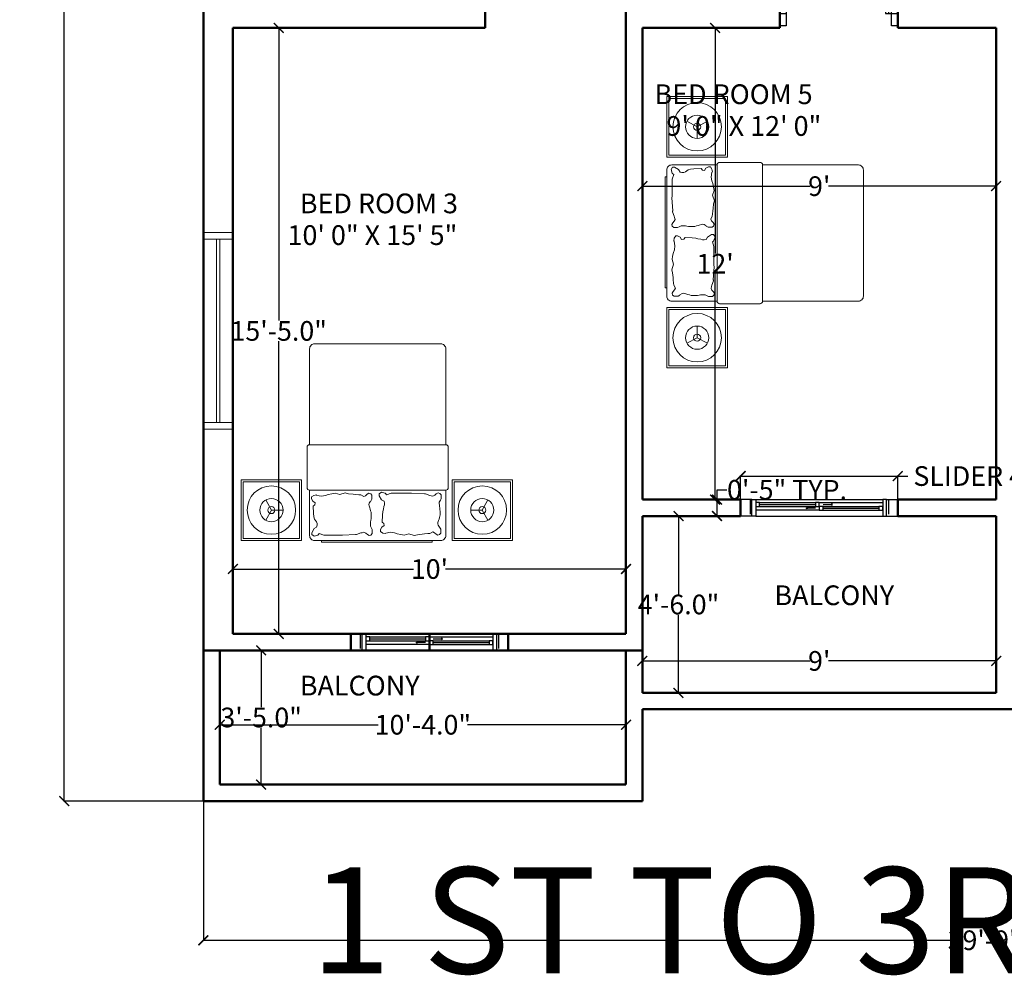
# Model space of a CAD drawing. Units: inches. Extents: x 147 to 1638, y 107 to 941.
# Tile 12 of 17: x 1062 to 1362, y 107 to 398. Entities that reach past the tile are written whole.
import ezdxf

# ---------------------------------------------------------------- set-up
doc = ezdxf.new("R2010")
doc.units = ezdxf.units.IN
doc.header["$MEASUREMENT"] = 0
for name, color, linetype, lineweight in [('A-ANNO-DIMS', 2, 'Continuous', 15), ('A-ANNO-TEXT', 7, 'Continuous', 25), ('A-AREA-IDEN', 7, 'Continuous', 18), ('A-Door', 150, 'Continuous', 25), ('furniture', 50, 'Continuous', 18), ('walls', 7, 'Continuous', 50), ('windows', 3, 'Continuous', 20)]:
    doc.layers.add(name, color=color, linetype=linetype, lineweight=lineweight)
doc.layers.add('A-Glaz', color=92, linetype='Continuous')
doc.layers.add('NT', color=1, linetype='Continuous')
doc.styles.get("Standard").update_dxf_attribs({"font": 'arial.ttf'})
doc.dimstyles.get("Standard").update_dxf_attribs({"dimtxt": 6, "dimasz": 3, "dimexe": 0.18, "dimexo": 0.0625, "dimgap": 0.09, "dimtad": 0, "dimtih": 1, "dimtoh": 1, "dimdec": 1, "dimzin": 0, "dimdsep": 46, "dimlunit": 3, "dimtxsty": 'Standard', "dimblk": 'ARCHTICK', "dimcen": 0.09, "dimadec": 0, "dimazin": 0, "dimtfac": 1, "dimtdec": 1, "dimtofl": 0, "dimtmove": 0, "dimatfit": 3, "dimfxl": 1, "dimtolj": 1, "dimtzin": 0, "dimarcsym": 0})

# ---------------------------------------------------------------- blocks, each defined once
blk = doc.blocks.new('A$C087A3AA9')
at = {"layer": 'A-Door'}
for points in [[(852.6, 94.7), (852.6, 852.6), (805.3, 852.6), (805.3, 94.7)], [(47.4, 94.7), (47.4, 0), (0, 0), (0, 94.7)], [(900, 94.7), (900, 0), (852.6, 0), (852.6, 94.7)]]:
    blk.add_lwpolyline(points, close=True, dxfattribs=at)
at = {"layer": 'A-Glaz'}
blk.add_line((828.9, 852.6), (828.9, 94.7), dxfattribs=at)
at = {"layer": 'NT'}
blk.add_arc((805.3, 94.7), 757.9, 90, 180, dxfattribs=at)
blk = doc.blocks.new('_ArchTick')
at = {"color": 0, "linetype": 'ByBlock', "const_width": 0.15}
blk.add_lwpolyline([(-0.5, -0.5), (0.5, 0.5)], dxfattribs=at)
blk = doc.blocks.new('*D34')
at = {"layer": 'A-ANNO-DIMS', "color": 0, "lineweight": -2, "transparency": 16777216}
for p, q in [((1266.83, 395.72), (1274.16, 395.72)), ((1273.98, 395.72), (1273.98, 326.82)), ((1273.98, 251.72), (1273.98, 320.62)), ((1266.83, 251.72), (1274.16, 251.72))]:
    blk.add_line(p, q, dxfattribs=at)
at = {"layer": 'Defpoints', "color": 0, "lineweight": -2, "transparency": 16777216}
for p in [(1266.77, 395.72), (1266.77, 251.72), (1273.98, 251.72)]:
    blk.add_point(p, dxfattribs=at)
at = {"layer": 'A-ANNO-DIMS', "color": 0, "lineweight": -2, "transparency": 16777216, "xscale": 3, "yscale": 3, "zscale": 3}
for p, rotation in [((1273.98, 395.72), 90), ((1273.98, 251.72), 270)]:
    blk.add_blockref('_ArchTick', p, dxfattribs=dict(at, rotation=rotation))
at = {"layer": 'A-ANNO-DIMS', "color": 0, "transparency": 16777216, "insert": (1273.98, 323.72), "char_height": 6, "attachment_point": 5}
blk.add_mtext("\\A1;12'", dxfattribs=at)
blk = doc.blocks.new('*D35')
at = {"layer": 'A-ANNO-DIMS', "color": 0, "lineweight": -2, "transparency": 16777216}
for p, q in [((1251.77, 336.12), (1251.77, 347.59)), ((1251.77, 347.41), (1302.92, 347.41)), ((1359.77, 347.41), (1308.62, 347.41)), ((1359.77, 336.12), (1359.77, 347.59))]:
    blk.add_line(p, q, dxfattribs=at)
at = {"layer": 'Defpoints', "color": 0, "lineweight": -2, "transparency": 16777216}
for p in [(1359.77, 347.41), (1251.77, 336.06), (1359.77, 336.06)]:
    blk.add_point(p, dxfattribs=at)
at = {"layer": 'A-ANNO-DIMS', "color": 0, "lineweight": -2, "transparency": 16777216, "xscale": 3, "yscale": 3, "zscale": 3, "rotation": 180}
blk.add_blockref('_ArchTick', (1251.77, 347.41), dxfattribs=at)
at = {"layer": 'A-ANNO-DIMS', "color": 0, "lineweight": -2, "transparency": 16777216, "xscale": 3, "yscale": 3, "zscale": 3}
blk.add_blockref('_ArchTick', (1359.77, 347.41), dxfattribs=at)
at = {"layer": 'A-ANNO-DIMS', "color": 0, "transparency": 16777216, "insert": (1305.77, 347.41), "char_height": 6, "attachment_point": 5}
blk.add_mtext("\\A1;9'", dxfattribs=at)
blk = doc.blocks.new('*D63')
at = {"layer": 'A-ANNO-DIMS', "color": 0, "lineweight": -2, "transparency": 16777216}
for p, q in [((1138.96, 395.72), (1140.94, 395.72)), ((1140.76, 395.72), (1140.76, 306.37)), ((1140.76, 210.72), (1140.76, 300.06)), ((1138.96, 210.72), (1140.94, 210.72))]:
    blk.add_line(p, q, dxfattribs=at)
at = {"layer": 'Defpoints', "color": 0, "lineweight": -2, "transparency": 16777216}
for p in [(1138.89, 395.72), (1138.89, 210.72), (1140.76, 210.72)]:
    blk.add_point(p, dxfattribs=at)
at = {"layer": 'A-ANNO-DIMS', "color": 0, "lineweight": -2, "transparency": 16777216, "xscale": 3, "yscale": 3, "zscale": 3}
for p, rotation in [((1140.76, 395.72), 90), ((1140.76, 210.72), 270)]:
    blk.add_blockref('_ArchTick', p, dxfattribs=dict(at, rotation=rotation))
at = {"layer": 'A-ANNO-DIMS', "color": 0, "transparency": 16777216, "insert": (1140.76, 303.22), "char_height": 6, "attachment_point": 5}
blk.add_mtext('\\A1;15\'-5.0"', dxfattribs=at)
blk = doc.blocks.new('*D64')
at = {"layer": 'A-ANNO-DIMS', "color": 0, "lineweight": -2, "transparency": 16777216}
for p, q in [((1126.77, 232.37), (1126.77, 230.36)), ((1246.77, 232.37), (1246.77, 230.36)), ((1126.77, 230.54), (1181.87, 230.54)), ((1246.77, 230.54), (1191.67, 230.54))]:
    blk.add_line(p, q, dxfattribs=at)
at = {"layer": 'Defpoints', "color": 0, "lineweight": -2, "transparency": 16777216}
for p in [(1126.77, 232.43), (1246.77, 232.43), (1246.77, 230.54)]:
    blk.add_point(p, dxfattribs=at)
at = {"layer": 'A-ANNO-DIMS', "color": 0, "lineweight": -2, "transparency": 16777216, "xscale": 3, "yscale": 3, "zscale": 3, "rotation": 180}
blk.add_blockref('_ArchTick', (1126.77, 230.54), dxfattribs=at)
at = {"layer": 'A-ANNO-DIMS', "color": 0, "lineweight": -2, "transparency": 16777216, "xscale": 3, "yscale": 3, "zscale": 3}
blk.add_blockref('_ArchTick', (1246.77, 230.54), dxfattribs=at)
at = {"layer": 'A-ANNO-DIMS', "color": 0, "transparency": 16777216, "insert": (1186.77, 230.54), "char_height": 6, "attachment_point": 5}
blk.add_mtext("\\A1;10'", dxfattribs=at)
blk = doc.blocks.new('*D67')
at = {"layer": 'A-ANNO-DIMS', "color": 0, "lineweight": -2, "transparency": 16777216}
for p, q in [((1122.77, 185.16), (1122.77, 182.83)), ((1246.77, 185.16), (1246.77, 182.83)), ((1122.77, 183.01), (1171.16, 183.01)), ((1246.77, 183.01), (1198.38, 183.01))]:
    blk.add_line(p, q, dxfattribs=at)
at = {"layer": 'Defpoints', "color": 0, "lineweight": -2, "transparency": 16777216}
for p in [(1122.77, 185.22), (1246.77, 185.22), (1246.77, 183.01)]:
    blk.add_point(p, dxfattribs=at)
at = {"layer": 'A-ANNO-DIMS', "color": 0, "lineweight": -2, "transparency": 16777216, "xscale": 3, "yscale": 3, "zscale": 3, "rotation": 180}
blk.add_blockref('_ArchTick', (1122.77, 183.01), dxfattribs=at)
at = {"layer": 'A-ANNO-DIMS', "color": 0, "lineweight": -2, "transparency": 16777216, "xscale": 3, "yscale": 3, "zscale": 3}
blk.add_blockref('_ArchTick', (1246.77, 183.01), dxfattribs=at)
at = {"layer": 'A-ANNO-DIMS', "color": 0, "transparency": 16777216, "insert": (1184.77, 183.01), "char_height": 6, "attachment_point": 5}
blk.add_mtext('\\A1;10\'-4.0"', dxfattribs=at)
blk = doc.blocks.new('*D68')
at = {"layer": 'A-ANNO-DIMS', "color": 0, "lineweight": -2, "transparency": 16777216}
for p, q in [((1132.43, 205.72), (1135.58, 205.72)), ((1135.4, 205.72), (1135.4, 188.37)), ((1135.4, 164.72), (1135.4, 182.06)), ((1132.43, 164.72), (1135.58, 164.72))]:
    blk.add_line(p, q, dxfattribs=at)
at = {"layer": 'Defpoints', "color": 0, "lineweight": -2, "transparency": 16777216}
for p in [(1132.37, 205.72), (1132.37, 164.72), (1135.4, 164.72)]:
    blk.add_point(p, dxfattribs=at)
at = {"layer": 'A-ANNO-DIMS', "color": 0, "lineweight": -2, "transparency": 16777216, "xscale": 3, "yscale": 3, "zscale": 3}
for p, rotation in [((1135.4, 205.72), 90), ((1135.4, 164.72), 270)]:
    blk.add_blockref('_ArchTick', p, dxfattribs=dict(at, rotation=rotation))
at = {"layer": 'A-ANNO-DIMS', "color": 0, "transparency": 16777216, "insert": (1135.4, 185.22), "char_height": 6, "attachment_point": 5}
blk.add_mtext('\\A1;3\'-5.0"', dxfattribs=at)
blk = doc.blocks.new('MAT-P14')
for p, q in [((-1.3369, 1.348), (-1.3369, 1.948)), ((-1.3369, 1.948), (-0.7369, 1.948)), ((-1.3169, 1.928), (-0.7569, 1.928)), ((-1.3169, 1.368), (-1.3169, 1.928)), ((-0.7569, 1.368), (-0.7569, 1.928)), ((-0.7369, 1.348), (-0.7369, 1.948)), ((0.625, 1.95), (-0.625, 1.95)), ((0.7534, 1.348), (0.7534, 1.948)), ((1.3534, 1.948), (0.7534, 1.948)), ((1.3334, 1.928), (0.7734, 1.928)), ((0.7734, 1.368), (0.7734, 1.928)), ((1.3334, 1.368), (1.3334, 1.928)), ((1.3534, 1.348), (1.3534, 1.948)), ((-1.0369, 1.648), (-1.0913, 1.7493)), ((1.0534, 1.648), (1.1078, 1.7493)), ((-1.0369, 1.648), (-1.0913, 1.5467)), ((-1.0369, 1.648), (-0.9219, 1.648)), ((1.0534, 1.648), (0.9384, 1.648)), ((1.0534, 1.648), (1.1078, 1.5467)), ((-1.3169, 1.368), (-0.7569, 1.368)), ((1.3334, 1.368), (0.7734, 1.368)), ((-1.3369, 1.348), (-0.7369, 1.348)), ((1.3534, 1.348), (0.7534, 1.348))]:
    blk.add_line(p, q)
blk.add_lwpolyline([(-0.5417, 1.95), (-0.5417, 1.9665), (0.5583, 1.9665), (0.5583, 1.95)], close=True)
for points in [[(-0.675, 1.45), (-0.675, 1.9, -0.414214), (-0.625, 1.95), (0.625, 1.95, -0.414214), (0.675, 1.9), (0.675, 1.45)], [(-0.675, 1, -0.414214), (-0.7, 1.025), (-0.7, 1.425, -0.414214), (-0.675, 1.45), (0.675, 1.45, -0.414214), (0.7, 1.425), (0.7, 1.025, -0.414214), (0.675, 1)], [(-0.625, 0, -0.414214), (-0.675, 0.05), (-0.675, 1), (0.675, 1), (0.675, 0.05, -0.414214), (0.625, 0)]]:
    blk.add_lwpolyline(points, format="xyb", close=True)
for points in [[(-0.6142, 1.8182), (-0.6262, 1.8377), (-0.6262, 1.8767), (-0.6142, 1.8914), (-0.5964, 1.8963), (-0.5785, 1.8865), (-0.563, 1.8719), (-0.5451, 1.8633), (-0.5157, 1.879), (-0.4966, 1.8816), (-0.4647, 1.8842), (-0.4393, 1.8868), (-0.3947, 1.892), (-0.3629, 1.8999), (-0.3094, 1.8823), (-0.2619, 1.8969), (-0.23, 1.8916), (-0.1918, 1.8838), (-0.1664, 1.8734), (-0.1282, 1.8682), (-0.0818, 1.8753), (-0.0758, 1.8802), (-0.052, 1.8753), (-0.0281, 1.8607), (-0.0281, 1.8412), (-0.0401, 1.8168), (-0.0639, 1.8022), (-0.0598, 1.781), (-0.0431, 1.7682), (-0.0463, 1.6973), (-0.0502, 1.6621), (-0.0561, 1.6397), (-0.0619, 1.6125), (-0.0678, 1.5965), (-0.0678, 1.5789), (-0.0631, 1.5599), (-0.0393, 1.5453), (-0.0147, 1.5053), (-0.0147, 1.4858), (-0.0385, 1.4711), (-0.0751, 1.4819), (-0.081, 1.4868), (-0.087, 1.4965), (-0.1344, 1.4812), (-0.3042, 1.4815), (-0.3178, 1.4815), (-0.3355, 1.4791), (-0.4636, 1.4878), (-0.4672, 1.4865), (-0.4732, 1.4863), (-0.5167, 1.5026), (-0.5299, 1.5053), (-0.5478, 1.5102), (-0.5656, 1.5015), (-0.5812, 1.4869), (-0.599, 1.4772), (-0.6169, 1.482), (-0.6288, 1.4967), (-0.6288, 1.5357), (-0.6229, 1.5503), (-0.611, 1.5698), (-0.6136, 1.6138), (-0.6149, 1.6269), (-0.6176, 1.6443), (-0.6189, 1.6595), (-0.6202, 1.6748), (-0.6202, 1.6955), (-0.6176, 1.7075), (-0.6136, 1.7227), (-0.6083, 1.7391), (-0.6043, 1.75), (-0.5976, 1.7707), (-0.5963, 1.7848), (-0.6003, 1.7979), (-0.6136, 1.8186)], [(0.0694, 1.5591), (0.0575, 1.5396), (0.0575, 1.5006), (0.0694, 1.4859), (0.0873, 1.481), (0.1052, 1.4908), (0.1207, 1.5054), (0.1386, 1.514), (0.168, 1.4983), (0.1871, 1.4957), (0.2189, 1.4931), (0.2444, 1.4905), (0.289, 1.4853), (0.3208, 1.4774), (0.3742, 1.495), (0.4218, 1.4804), (0.4536, 1.4857), (0.4918, 1.4935), (0.5173, 1.5039), (0.5555, 1.5091), (0.6019, 1.502), (0.6079, 1.4971), (0.6317, 1.502), (0.6555, 1.5166), (0.6555, 1.5361), (0.6436, 1.5605), (0.6198, 1.5751), (0.6239, 1.5963), (0.6405, 1.6091), (0.6373, 1.68), (0.6334, 1.7152), (0.6276, 1.7376), (0.6063, 1.7648), (0.6005, 1.7808), (0.6005, 1.7984), (0.6051, 1.8174), (0.6289, 1.832), (0.6536, 1.872), (0.6536, 1.8915), (0.6298, 1.9062), (0.5932, 1.8954), (0.5872, 1.8905), (0.5813, 1.8808), (0.5338, 1.8961), (0.3795, 1.8958), (0.3658, 1.8958), (0.3482, 1.8982), (0.2201, 1.8895), (0.2165, 1.8908), (0.2104, 1.891), (0.1669, 1.8747), (0.1538, 1.872), (0.1359, 1.8671), (0.118, 1.8758), (0.1025, 1.8904), (0.0846, 1.9001), (0.0667, 1.8953), (0.0548, 1.8806), (0.0548, 1.8416), (0.0608, 1.827), (0.0727, 1.8075), (0.0701, 1.7635), (0.0688, 1.7504), (0.0661, 1.733), (0.0648, 1.7178), (0.0634, 1.7025), (0.0634, 1.6818), (0.0661, 1.6698), (0.0701, 1.6546), (0.0754, 1.6382), (0.0794, 1.6273), (0.086, 1.6066), (0.0874, 1.5925), (0.0834, 1.5794), (0.0701, 1.5587)]]:
    blk.add_lwpolyline(points)
for centre, radius in [((-1.0369, 1.648), 0.24), ((1.0534, 1.648), 0.24), ((-1.0369, 1.648), 0.115), ((1.0534, 1.648), 0.115), ((-1.0369, 1.648), 0.035), ((1.0534, 1.648), 0.035)]:
    blk.add_circle(centre, radius)
blk = doc.blocks.new('*D83')
at = {"layer": 'A-ANNO-DIMS', "color": 0, "lineweight": -2, "transparency": 16777216}
for p, q in [((1261.96, 246.72), (1262.99, 246.72)), ((1262.81, 246.72), (1262.81, 222.87)), ((1262.81, 192.72), (1262.81, 216.56)), ((1261.96, 192.72), (1262.99, 192.72))]:
    blk.add_line(p, q, dxfattribs=at)
at = {"layer": 'Defpoints', "color": 0, "lineweight": -2, "transparency": 16777216}
for p in [(1261.89, 246.72), (1261.89, 192.72), (1262.81, 192.72)]:
    blk.add_point(p, dxfattribs=at)
at = {"layer": 'A-ANNO-DIMS', "color": 0, "lineweight": -2, "transparency": 16777216, "xscale": 3, "yscale": 3, "zscale": 3}
for p, rotation in [((1262.81, 246.72), 90), ((1262.81, 192.72), 270)]:
    blk.add_blockref('_ArchTick', p, dxfattribs=dict(at, rotation=rotation))
at = {"layer": 'A-ANNO-DIMS', "color": 0, "transparency": 16777216, "insert": (1262.81, 219.72), "char_height": 6, "attachment_point": 5}
blk.add_mtext('\\A1;4\'-6.0"', dxfattribs=at)
blk = doc.blocks.new('*D84')
at = {"layer": 'A-ANNO-DIMS', "color": 0, "lineweight": -2, "transparency": 16777216}
for p, q in [((1251.77, 199.83), (1251.77, 202.67)), ((1251.77, 202.49), (1302.92, 202.49)), ((1359.77, 202.49), (1308.62, 202.49)), ((1359.77, 199.83), (1359.77, 202.67))]:
    blk.add_line(p, q, dxfattribs=at)
at = {"layer": 'Defpoints', "color": 0, "lineweight": -2, "transparency": 16777216}
for p in [(1359.77, 202.49), (1251.77, 199.77), (1359.77, 199.77)]:
    blk.add_point(p, dxfattribs=at)
at = {"layer": 'A-ANNO-DIMS', "color": 0, "lineweight": -2, "transparency": 16777216, "xscale": 3, "yscale": 3, "zscale": 3, "rotation": 180}
blk.add_blockref('_ArchTick', (1251.77, 202.49), dxfattribs=at)
at = {"layer": 'A-ANNO-DIMS', "color": 0, "lineweight": -2, "transparency": 16777216, "xscale": 3, "yscale": 3, "zscale": 3}
blk.add_blockref('_ArchTick', (1359.77, 202.49), dxfattribs=at)
at = {"layer": 'A-ANNO-DIMS', "color": 0, "transparency": 16777216, "insert": (1305.77, 202.49), "char_height": 6, "attachment_point": 5}
blk.add_mtext("\\A1;9'", dxfattribs=at)
blk = doc.blocks.new('WIN-60IN')
for p, q in [((60, 9), (0, 9)), ((0, 9), (0, 0)), ((2, 9), (2, 0)), ((58, 0), (58, 9)), ((60, 0), (60, 9)), ((2, 5), (58, 5)), ((2, 4), (58, 4)), ((0, 0), (60, 0))]:
    blk.add_line(p, q)
blk = doc.blocks.new('DOOR-SLIDING-48IN')
for p, q in [((3.46, 5), (0, 5)), ((2.87, 5), (2.87, 0.59)), ((3.46, 0), (3.46, 5)), ((3.46, 5), (4.63, 5)), ((4.63, 5), (43.37, 5)), ((4.63, 5), (4.63, 0)), ((5.81, 4.11), (22.83, 4.11)), ((5.81, 3.52), (22.83, 3.52)), ((24, 4.11), (43.37, 4.11)), ((25.17, 3.52), (27.7, 3.52)), ((44.54, 5), (43.37, 5)), ((43.37, 5), (43.37, 0)), ((44.54, 5), (48, 5)), ((44.54, 0), (44.54, 5)), ((45.13, 5), (45.13, 0.59)), ((3.46, 0), (0, 0)), ((4.63, 0), (3.46, 0)), ((24, 1.76), (4.63, 1.76)), ((4.63, 0), (43.37, 0)), ((5.81, 2.93), (22.83, 2.93)), ((22.83, 2.35), (20.3, 2.35)), ((25.17, 2.93), (42.19, 2.93)), ((25.17, 2.35), (42.19, 2.35)), ((25.17, 1.76), (42.19, 1.76)), ((43.37, 0), (44.54, 0)), ((44.54, 0), (48, 0))]:
    blk.add_line(p, q)
for points in [[(4.63, 2.93), (5.81, 2.93), (5.81, 4.11), (4.63, 4.11)], [(22.83, 2.93), (24, 2.93), (24, 4.11), (22.83, 4.11)], [(28, 3.52), (27.7, 3.7), (27.7, 3.35)], [(20, 2.35), (20.3, 2.52), (20.3, 2.17)], [(24, 1.76), (25.17, 1.76), (25.17, 2.93), (24, 2.93)], [(42.19, 1.76), (43.37, 1.76), (43.37, 2.93), (42.19, 2.93)]]:
    blk.add_lwpolyline(points, close=True)
blk = doc.blocks.new('*D108')
at = {"layer": 'A-ANNO-DIMS', "color": 0, "lineweight": -2, "transparency": 16777216}
for p, q in [((1281.77, 251.78), (1281.77, 259.1)), ((1281.77, 258.92), (1329.77, 258.92)), ((1329.77, 251.78), (1329.77, 259.1)), ((1329.77, 258.92), (1332.77, 258.92))]:
    blk.add_line(p, q, dxfattribs=at)
at = {"layer": 'Defpoints', "color": 0, "lineweight": -2, "transparency": 16777216}
for p in [(1329.77, 258.92), (1281.77, 251.72), (1329.77, 251.72)]:
    blk.add_point(p, dxfattribs=at)
at = {"layer": 'A-ANNO-DIMS', "color": 0, "lineweight": -2, "transparency": 16777216, "xscale": 3, "yscale": 3, "zscale": 3, "rotation": 180}
blk.add_blockref('_ArchTick', (1281.77, 258.92), dxfattribs=at)
at = {"layer": 'A-ANNO-DIMS', "color": 0, "lineweight": -2, "transparency": 16777216, "xscale": 3, "yscale": 3, "zscale": 3}
blk.add_blockref('_ArchTick', (1329.77, 258.92), dxfattribs=at)
at = {"layer": 'A-ANNO-DIMS', "color": 0, "transparency": 16777216, "insert": (1367.43, 258.92), "char_height": 6, "attachment_point": 5}
blk.add_mtext('\\A1;SLIDER 4\'-0" TYP.', dxfattribs=at)
blk = doc.blocks.new('*D109')
at = {"layer": 'A-ANNO-DIMS', "color": 0, "lineweight": -2, "transparency": 16777216}
for p, q in [((1274.57, 251.72), (1274.57, 254.72)), ((1274.57, 254.72), (1277.57, 254.72)), ((1281.71, 251.72), (1274.39, 251.72)), ((1274.57, 246.72), (1274.57, 251.72)), ((1281.71, 246.72), (1274.39, 246.72))]:
    blk.add_line(p, q, dxfattribs=at)
at = {"layer": 'Defpoints', "color": 0, "lineweight": -2, "transparency": 16777216}
for p in [(1274.57, 251.72), (1281.77, 251.72), (1281.77, 246.72)]:
    blk.add_point(p, dxfattribs=at)
at = {"layer": 'A-ANNO-DIMS', "color": 0, "lineweight": -2, "transparency": 16777216, "xscale": 3, "yscale": 3, "zscale": 3}
for p, rotation in [((1274.57, 251.72), 90), ((1274.57, 246.72), 270)]:
    blk.add_blockref('_ArchTick', p, dxfattribs=dict(at, rotation=rotation))
at = {"layer": 'A-ANNO-DIMS', "color": 0, "transparency": 16777216, "insert": (1295.94, 254.72), "char_height": 6, "attachment_point": 5}
blk.add_mtext('\\A1;0\'-5" TYP.', dxfattribs=at)
blk = doc.blocks.new('*D134')
at = {"layer": 'A-ANNO-DIMS', "color": 0, "lineweight": -2, "transparency": 16777216}
for p, q in [((1117.77, 159.66), (1117.77, 117.04)), ((1594.77, 159.66), (1594.77, 117.04)), ((1117.77, 117.22), (1345.87, 117.22)), ((1594.77, 117.22), (1366.66, 117.22))]:
    blk.add_line(p, q, dxfattribs=at)
at = {"layer": 'Defpoints', "color": 0, "lineweight": -2, "transparency": 16777216}
for p in [(1117.77, 159.72), (1594.77, 159.72), (1594.77, 117.22)]:
    blk.add_point(p, dxfattribs=at)
at = {"layer": 'A-ANNO-DIMS', "color": 0, "lineweight": -2, "transparency": 16777216, "xscale": 3, "yscale": 3, "zscale": 3, "rotation": 180}
blk.add_blockref('_ArchTick', (1117.77, 117.22), dxfattribs=at)
at = {"layer": 'A-ANNO-DIMS', "color": 0, "lineweight": -2, "transparency": 16777216, "xscale": 3, "yscale": 3, "zscale": 3}
blk.add_blockref('_ArchTick', (1594.77, 117.22), dxfattribs=at)
at = {"layer": 'A-ANNO-DIMS', "color": 0, "transparency": 16777216, "insert": (1356.27, 117.22), "char_height": 6, "attachment_point": 5}
blk.add_mtext('\\A1;39\'-9"', dxfattribs=at)
blk = doc.blocks.new('*D135')
at = {"layer": 'A-ANNO-DIMS', "color": 0, "lineweight": -2, "transparency": 16777216}
for p, q in [((1176.71, 938.72), (1075.09, 938.72)), ((1075.27, 938.72), (1075.27, 552.37)), ((1075.27, 159.72), (1075.27, 546.06)), ((1117.71, 159.72), (1075.09, 159.72))]:
    blk.add_line(p, q, dxfattribs=at)
at = {"layer": 'Defpoints', "color": 0, "lineweight": -2, "transparency": 16777216}
for p in [(1075.27, 938.72), (1176.77, 938.72), (1117.77, 159.72)]:
    blk.add_point(p, dxfattribs=at)
at = {"layer": 'A-ANNO-DIMS', "color": 0, "lineweight": -2, "transparency": 16777216, "xscale": 3, "yscale": 3, "zscale": 3}
for p, rotation in [((1075.27, 938.72), 90), ((1075.27, 159.72), 270)]:
    blk.add_blockref('_ArchTick', p, dxfattribs=dict(at, rotation=rotation))
at = {"layer": 'A-ANNO-DIMS', "color": 0, "transparency": 16777216, "insert": (1075.27, 549.22), "char_height": 6, "attachment_point": 5}
blk.add_mtext('\\A1;64\'-11"', dxfattribs=at)

msp = doc.modelspace()

# ---------------------------------------------------------------- linework, layer by layer
at = {"layer": 'walls'}
for p, q in [((1117.77, 909.72), (1117.77, 201.72)), ((1203.77, 448.72), (1203.77, 395.72)), ((1246.77, 436.72), (1246.77, 210.72)), ((1293.77, 400.72), (1293.77, 395.72)), ((1329.77, 400.72), (1329.77, 395.72)), ((1126.77, 395.72), (1126.77, 210.72)), ((1126.77, 395.72), (1203.77, 395.72)), ((1251.77, 395.72), (1251.77, 251.72)), ((1251.77, 395.72), (1281.77, 395.72)), ((1293.77, 395.72), (1281.77, 395.72)), ((1329.77, 395.72), (1359.77, 395.72)), ((1359.77, 395.72), (1359.77, 251.72)), ((1251.77, 251.72), (1281.77, 251.72)), ((1281.77, 246.72), (1281.77, 251.72)), ((1329.77, 251.72), (1359.77, 251.72)), ((1329.77, 246.72), (1329.77, 251.72)), ((1251.77, 246.72), (1251.77, 192.72)), ((1251.77, 246.72), (1281.77, 246.72)), ((1329.77, 246.72), (1359.77, 246.72)), ((1359.77, 246.72), (1359.77, 192.72)), ((1246.77, 210.72), (1126.77, 210.72)), ((1162.77, 205.72), (1162.77, 210.72)), ((1186.77, 210.72), (1186.77, 205.72)), ((1210.77, 205.72), (1210.77, 210.72)), ((1251.77, 205.72), (1117.77, 205.72)), ((1122.77, 205.72), (1122.77, 164.72)), ((1246.77, 205.72), (1246.77, 164.72)), ((1117.77, 201.72), (1117.77, 159.72)), ((1251.77, 192.72), (1359.77, 192.72)), ((1251.77, 187.72), (1460.77, 187.72)), ((1251.77, 187.72), (1251.77, 159.72)), ((1122.77, 164.72), (1246.77, 164.72)), ((1117.77, 159.72), (1251.77, 159.72))]:
    msp.add_line(p, q, dxfattribs=at)

# ---------------------------------------------------------------- block references
at = {"layer": 'A-Door', "xscale": 0.0400000000000001, "yscale": 0.0400000000000001, "zscale": 0.0400000000000001}
msp.add_blockref('A$C087A3AA9', (1293.77, 396.32), dxfattribs=at)
at = {"layer": 'A-Door'}
for p in [(1281.77, 246.72), (1162.77, 205.72)]:
    msp.add_blockref('DOOR-SLIDING-48IN', p, dxfattribs=at)
at = {"layer": 'furniture', "xscale": 30.80045642108221, "yscale": 30.80045642108221, "zscale": 30.80045642108221}
for p, rotation in [((1319.26, 333.09), 89.99999999999999), ((1170.97, 299.29), 180)]:
    msp.add_blockref('MAT-P14', p, dxfattribs=dict(at, rotation=rotation))
at = {"layer": 'windows', "rotation": 270.0000000000011}
msp.add_blockref('WIN-60IN', (1117.77, 333.22), dxfattribs=at)

# ---------------------------------------------------------------- texts
at = {"layer": 'A-ANNO-TEXT'}
msp.add_text('1 ST TO 3RD FLOORS', height=32.387, dxfattribs=at).set_placement((1150.48, 107.1))
at = {"layer": 'A-AREA-IDEN'}
for s, height, p in [('BED ROOM 5', 6.031, (1255.47, 372.45)), ('9\' 0" X 12\' 0"', 6.0306, (1259.12, 362.76)), ('BED ROOM 3', 6.031, (1147.2, 339.13)), ('  10\' 0" X 15\' 5"', 6.0306, (1139.75, 329.45)), ('BALCONY', 6.031, (1292.08, 219.51)), ('BALCONY', 6.031, (1147.2, 191.94))]:
    msp.add_text(s, height=height, dxfattribs=at).set_placement(p)

# ---------------------------------------------------------------- dimensions: what is measured, and where the dimension line sits
at = {"layer": 'A-ANNO-DIMS'}
for base, p1, p2, override, picture, middle in [((1075.27, 938.72), (1117.77, 159.72), (1176.77, 938.72), {"dimdec": 1, "dimlfac": 1, "dimrnd": 0, "dimzin": 1, "dimdsep": 46, "dimlunit": 4, "dimfrac": 2}, '*D135', (1075.27, 549.22)), ((1140.76, 210.72), (1138.89, 395.72), (1138.89, 210.72), {"dimclrd": 0, "dimclre": 0, "dimclrt": 0}, '*D63', (1140.76, 303.22)), ((1273.98, 251.72), (1266.77, 395.72), (1266.77, 251.72), {"dimclrd": 0, "dimclre": 0, "dimclrt": 0}, '*D34', (1273.98, 323.72)), ((1262.81, 192.72), (1261.89, 246.72), (1261.89, 192.72), {"dimclrd": 0, "dimclre": 0, "dimclrt": 0}, '*D83', (1262.81, 219.72)), ((1135.4, 164.72), (1132.37, 205.72), (1132.37, 164.72), {"dimclrd": 0, "dimclre": 0, "dimclrt": 0}, '*D68', (1135.4, 185.22))]:
    dim = msp.add_linear_dim(base=base, p1=p1, p2=p2, angle=90, dimstyle='Standard', override=override, dxfattribs=at)
    dim.commit()
    dim.dimension.update_dxf_attribs({"geometry": picture, "text_midpoint": middle})
for base, p1, p2, override, picture, middle in [((1359.77, 347.41), (1251.77, 336.06), (1359.77, 336.06), {"dimclrd": 0, "dimclre": 0, "dimclrt": 0}, '*D35', (1305.77, 347.41)), ((1246.77, 230.54), (1126.77, 232.43), (1246.77, 232.43), {"dimclrd": 0, "dimclre": 0, "dimclrt": 0}, '*D64', (1186.77, 230.54)), ((1359.77, 202.49), (1251.77, 199.77), (1359.77, 199.77), {"dimclrd": 0, "dimclre": 0, "dimclrt": 0}, '*D84', (1305.77, 202.49)), ((1246.77, 183.01), (1122.77, 185.22), (1246.77, 185.22), {"dimclrd": 0, "dimclre": 0, "dimclrt": 0}, '*D67', (1184.77, 183.01)), ((1594.77, 117.22), (1117.77, 159.72), (1594.77, 159.72), {"dimdec": 1, "dimlfac": 1, "dimrnd": 0, "dimzin": 1, "dimdsep": 46, "dimlunit": 4, "dimfrac": 2}, '*D134', (1356.27, 117.22))]:
    dim = msp.add_linear_dim(base=base, p1=p1, p2=p2, dimstyle='Standard', override=override, dxfattribs=at)
    dim.commit()
    dim.dimension.update_dxf_attribs({"geometry": picture, "text_midpoint": middle})
dim = msp.add_linear_dim(base=(1329.77, 258.92), p1=(1281.77, 251.72), p2=(1329.77, 251.72), text='SLIDER <> TYP.', dimstyle='Standard', override={"dimdec": 1, "dimlfac": 1, "dimrnd": 0, "dimzin": 1, "dimdsep": 46, "dimlunit": 4, "dimfrac": 2}, dxfattribs=at)
dim.commit()
dim.dimension.update_dxf_attribs({"geometry": '*D108', "text_midpoint": (1367.43, 258.92)})
dim = msp.add_linear_dim(base=(1274.57, 251.72), p1=(1281.77, 246.72), p2=(1281.77, 251.72), angle=90, text='<> TYP.', dimstyle='Standard', override={"dimdec": 1, "dimlfac": 1, "dimrnd": 0, "dimzin": 1, "dimdsep": 46, "dimlunit": 4, "dimfrac": 2}, dxfattribs=at)
dim.commit()
dim.dimension.update_dxf_attribs({"geometry": '*D109', "text_midpoint": (1295.94, 254.72)})

doc.saveas('drawing.dxf')
